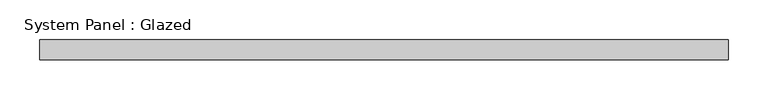
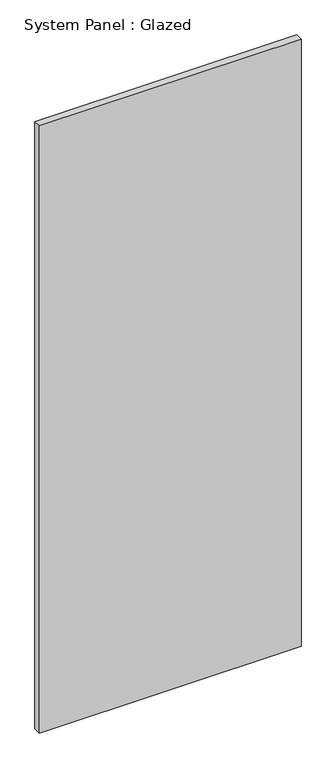
"""IFC4 building model written with IfcOpenShell, lengths in millimetres: plate geometry, System Panel : Glazed."""

from ifc_helpers import new_model, si_unit, origin, origin_with_axes, place, context, project, spatial, polyline, outline, extrude, source, transform, mapped, element, save


def system_panel_glazed_c09e287b(model_context):
    return source(origin(), model_context, "Body", "SweptSolid", [
        extrude(outline(polyline([(432.2, 24.5), (-432.2, 24.5), (-432.2, 49.5), (432.2, 49.5), (432.2, 24.5)])), origin_with_axes(), (0.0, 0.0, 1.0), 2119.3021954),
    ])


if __name__ == "__main__":
    model = new_model("IFC4")
    model_context = context("Model", 3, world=origin())
    ifc_project = project(units=[si_unit("LENGTHUNIT", "METRE", prefix="MILLI")], contexts=[model_context])
    site = spatial("IfcSite", under=ifc_project)
    building = spatial("IfcBuilding", under=site)
    placement = place(None, origin())
    system_panel_glazed_shape = system_panel_glazed_c09e287b(model_context)
    element("IfcPlate", 1, ObjectType="System Panel : Glazed", at=placement, inside=building, context=model_context, shape_type="MappedRepresentation", body=[
        mapped(system_panel_glazed_shape, transform((0.0, 0.0, 0.0), x_axis=(1.0, 0.0, 0.0), y_axis=(0.0, 1.0, 0.0), z_axis=(0.0, 0.0, 1.0))),
    ])
    save(model, "model.ifc")

# Revit data of these elements
# Type "System Panel : Glazed"
#   Keynote = "H11"
#   Construction Type Id = "GSP4R"
#   Analytic Construction = "1/8 in Pilkington single glazing"
#   Visual Light Transmittance = 0.9
#   Solar Heat Gain Coefficient = 0.86
#   Heat Transfer Coefficient (U) = 6.7069 W/(m²·K)
#   Define Thermal Properties by = 1
# Element 1 (IfcPlate, "System Panel : Glazed")
#   Materials on its faces: "Glass"
# Materials
#   "Glass": class "Glass", colour RGB 0 128 192, transparency 0.9, Description = "Soda Lime Glass", Cost = 0
